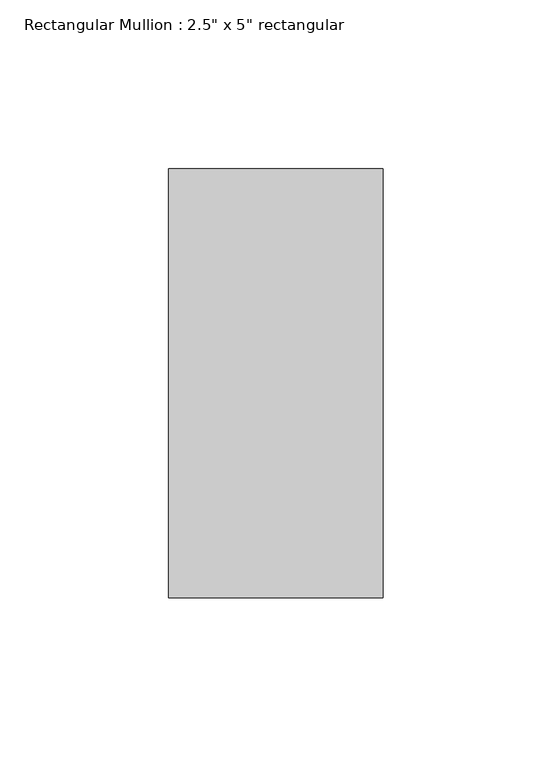
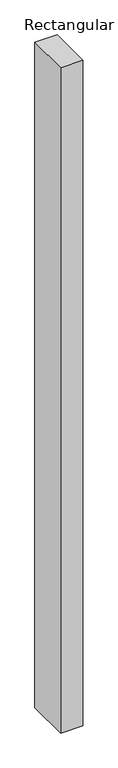
"""IFC4 building model written with IfcOpenShell, lengths in millimetres: member geometry."""

from ifc_helpers import new_model, si_unit, frame, origin, place, context, project, spatial, polyline, outline, extrude, source, transform, mapped, element, save


def member_16b81337(model_context):
    return source(origin(), model_context, "Body", "SweptSolid", [
        extrude(outline(polyline([(0.0, 63.5), (0.0, -63.5), (-63.5, -63.5), (-63.5, 63.5), (0.0, 63.5)])), frame((0.0, 0.0, -2006.6), z_axis=(0.0, 0.0, 1.0), x_axis=(1.0, 0.0, 0.0)), (0.0, 0.0, 1.0), 2006.6),
    ])


if __name__ == "__main__":
    model = new_model("IFC4")
    model_context = context("Model", 3, world=origin())
    ifc_project = project(units=[si_unit("LENGTHUNIT", "METRE", prefix="MILLI")], contexts=[model_context])
    site = spatial("IfcSite", under=ifc_project)
    building = spatial("IfcBuilding", under=site)
    placement = place(None, origin())
    member_shape = member_16b81337(model_context)
    element("IfcMember", 1, ObjectType="Rectangular Mullion : 2.5\" x 5\" rectangular", at=placement, inside=building, context=model_context, shape_type="MappedRepresentation", body=[
        mapped(member_shape, transform((0.0, 0.0, 0.0), x_axis=(1.0, 0.0, 0.0), y_axis=(0.0, 1.0, 0.0), z_axis=(0.0, 0.0, 1.0))),
    ])
    save(model, "model.ifc")

# Revit data of these elements
# Type "Rectangular Mullion : 2.5\" x 5\" rectangular"
#   built-in parameter 1007304 = 0.416667 (stored number, unit not read)
#   built-in parameter 1007301 = 0.104167 (stored number, unit not read)
#   built-in parameter 1007300 = 0.104167 (stored number, unit not read)
# Element 1 (IfcMember, "Rectangular Mullion : 2.5\" x 5\" rectangular")
#   Materials on its faces: "Aluminum"
# Materials
#   "Aluminum": class "Metal", colour RGB 247 247 247, transparency 0, Description = "Aluminum 6061", Cost = 0
